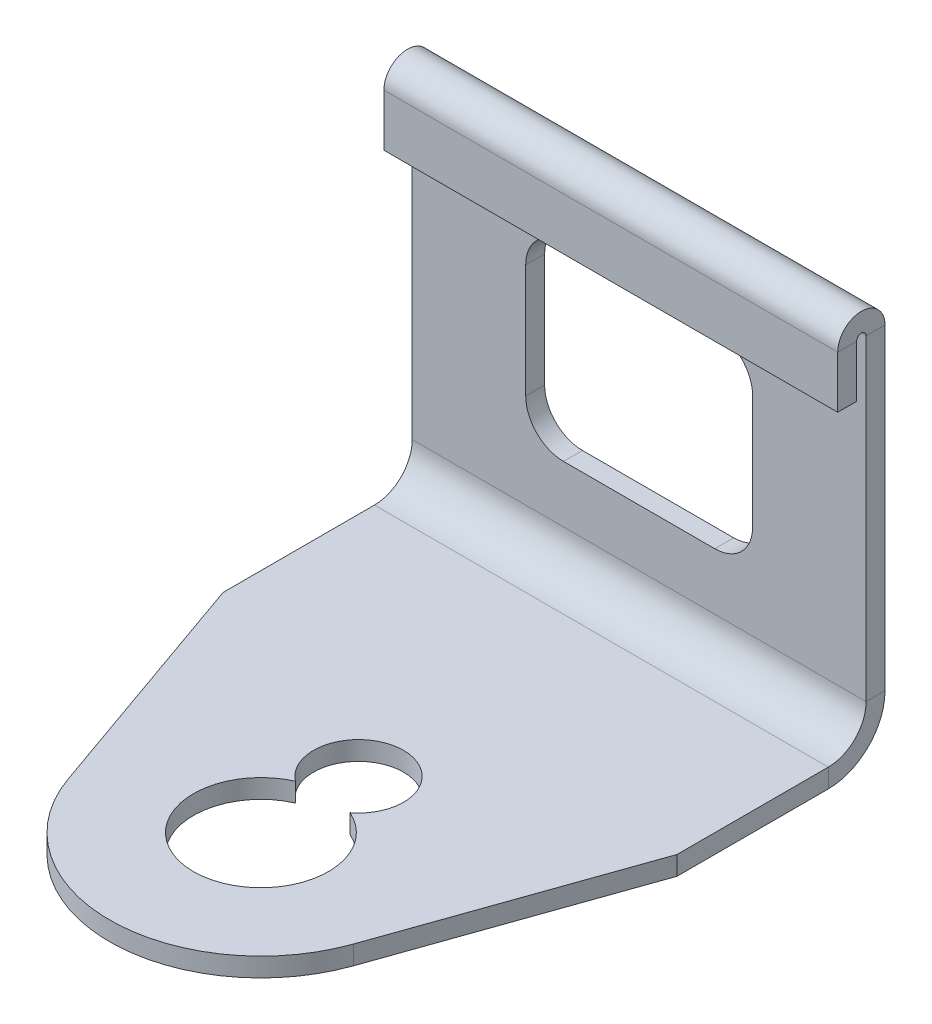
ISO-10303-21;
HEADER;
FILE_DESCRIPTION(('STEP AP214'),'2;1');
FILE_NAME('part.step','',(''),(''),'','','');
FILE_SCHEMA(('AUTOMOTIVE_DESIGN { 1 0 10303 214 1 1 1 1 }'));
ENDSEC;
DATA;
#1=APPLICATION_CONTEXT('core data for automotive mechanical design processes');
#2=APPLICATION_PROTOCOL_DEFINITION('international standard','automotive_design',2000,#1);
#3=PRODUCT_CONTEXT('',#1,'mechanical');
#4=PRODUCT('Part','Part','',(#3));
#5=PRODUCT_RELATED_PRODUCT_CATEGORY('part','',(#4));
#6=PRODUCT_DEFINITION_FORMATION('','',#4);
#7=PRODUCT_DEFINITION_CONTEXT('part definition',#1,'design');
#8=PRODUCT_DEFINITION('design','',#6,#7);
#9=PRODUCT_DEFINITION_SHAPE('','',#8);
#10=(LENGTH_UNIT() NAMED_UNIT(*) SI_UNIT(.MILLI.,.METRE.));
#11=(NAMED_UNIT(*) PLANE_ANGLE_UNIT() SI_UNIT($,.RADIAN.));
#12=(NAMED_UNIT(*) SI_UNIT($,.STERADIAN.) SOLID_ANGLE_UNIT());
#13=UNCERTAINTY_MEASURE_WITH_UNIT(LENGTH_MEASURE(1.E-05),#10,'distance_accuracy_value','');
#14=(GEOMETRIC_REPRESENTATION_CONTEXT(3) GLOBAL_UNCERTAINTY_ASSIGNED_CONTEXT((#13)) GLOBAL_UNIT_ASSIGNED_CONTEXT((#10,
#11,#12)) REPRESENTATION_CONTEXT('',''));
#15=CARTESIAN_POINT('',(0.,0.,0.));
#16=DIRECTION('',(0.,0.,1.));
#17=DIRECTION('',(1.,0.,0.));
#18=AXIS2_PLACEMENT_3D('',#15,#16,#17);
#19=CARTESIAN_POINT('',(-12.,-1.,11.));
#20=DIRECTION('',(-1.,0.,0.));
#21=DIRECTION('',(0.,0.,1.));
#22=AXIS2_PLACEMENT_3D('',#19,#20,#21);
#23=PLANE('',#22);
#24=DIRECTION('',(0.,0.,1.));
#25=VECTOR('',#24,1.);
#26=CARTESIAN_POINT('',(-12.,0.,11.));
#27=LINE('',#26,#25);
#28=CARTESIAN_POINT('',(-12.,0.,2.99999999999999));
#29=VERTEX_POINT('',#28);
#30=CARTESIAN_POINT('',(-12.,0.,11.));
#31=VERTEX_POINT('',#30);
#32=EDGE_CURVE('E463',#29,#31,#27,.T.);
#33=ORIENTED_EDGE('',*,*,#32,.F.);
#34=DIRECTION('',(0.,-1.,0.));
#35=VECTOR('',#34,1.);
#36=CARTESIAN_POINT('',(-12.,0.,2.99999999999999));
#37=LINE('',#36,#35);
#38=CARTESIAN_POINT('',(-12.,-1.00000000000002,2.99999999999999));
#39=VERTEX_POINT('',#38);
#40=EDGE_CURVE('E412',#29,#39,#37,.T.);
#41=ORIENTED_EDGE('',*,*,#40,.T.);
#42=DIRECTION('',(0.,0.,1.));
#43=VECTOR('',#42,1.);
#44=CARTESIAN_POINT('',(-12.,-1.,11.));
#45=LINE('',#44,#43);
#46=CARTESIAN_POINT('',(-12.,-1.,11.));
#47=VERTEX_POINT('',#46);
#48=EDGE_CURVE('E446',#39,#47,#45,.T.);
#49=ORIENTED_EDGE('',*,*,#48,.T.);
#50=DIRECTION('',(0.,1.,0.));
#51=VECTOR('',#50,1.);
#52=CARTESIAN_POINT('',(-12.,-1.,11.));
#53=LINE('',#52,#51);
#54=EDGE_CURVE('E97',#47,#31,#53,.T.);
#55=ORIENTED_EDGE('',*,*,#54,.T.);
#56=EDGE_LOOP('',(#33,#41,#49,#55));
#57=FACE_BOUND('',#56,.T.);
#58=ADVANCED_FACE('F92',(#57),#23,.T.);
#59=CARTESIAN_POINT('',(0.,-1.,21.));
#60=DIRECTION('',(0.,1.,0.));
#61=DIRECTION('',(0.,0.,1.));
#62=AXIS2_PLACEMENT_3D('',#59,#60,#61);
#63=PLANE('',#62);
#64=CARTESIAN_POINT('',(0.,-1.,15.84));
#65=DIRECTION('',(0.,1.,0.));
#66=DIRECTION('',(0.,0.,1.));
#67=AXIS2_PLACEMENT_3D('',#64,#65,#66);
#68=CIRCLE('',#67,2.38);
#69=CARTESIAN_POINT('',(1.44136175339873,-1.,17.7339050387597));
#70=VERTEX_POINT('',#69);
#71=CARTESIAN_POINT('',(-1.44136175339873,-1.,17.7339050387597));
#72=VERTEX_POINT('',#71);
#73=EDGE_CURVE('E435',#70,#72,#68,.T.);
#74=ORIENTED_EDGE('',*,*,#73,.T.);
#75=CARTESIAN_POINT('',(0.,-1.,21.));
#76=DIRECTION('',(0.,1.,0.));
#77=DIRECTION('',(0.,0.,1.));
#78=AXIS2_PLACEMENT_3D('',#75,#76,#77);
#79=CIRCLE('',#78,3.57);
#80=EDGE_CURVE('E427',#72,#70,#79,.T.);
#81=ORIENTED_EDGE('',*,*,#80,.T.);
#82=EDGE_LOOP('',(#74,#81));
#83=FACE_BOUND('',#82,.T.);
#84=DIRECTION('',(-1.,0.,0.));
#85=VECTOR('',#84,1.);
#86=CARTESIAN_POINT('',(-12.,-1.00000000000002,2.99999999999999));
#87=LINE('',#86,#85);
#88=CARTESIAN_POINT('',(12.,-1.,2.99999999999999));
#89=VERTEX_POINT('',#88);
#90=EDGE_CURVE('E406',#39,#89,#87,.F.);
#91=ORIENTED_EDGE('',*,*,#90,.T.);
#92=DIRECTION('',(0.,0.,-1.));
#93=VECTOR('',#92,1.);
#94=CARTESIAN_POINT('',(12.,-1.,11.));
#95=LINE('',#94,#93);
#96=CARTESIAN_POINT('',(12.,-1.,11.));
#97=VERTEX_POINT('',#96);
#98=EDGE_CURVE('E443',#97,#89,#95,.T.);
#99=ORIENTED_EDGE('',*,*,#98,.F.);
#100=DIRECTION('',(0.331954485163873,0.,-0.943295404303227));
#101=VECTOR('',#100,1.);
#102=CARTESIAN_POINT('',(12.,-1.,11.));
#103=LINE('',#102,#101);
#104=CARTESIAN_POINT('',(7.54636323442581,-1.,23.655635881311));
#105=VERTEX_POINT('',#104);
#106=EDGE_CURVE('E460',#105,#97,#103,.T.);
#107=ORIENTED_EDGE('',*,*,#106,.F.);
#108=CARTESIAN_POINT('',(0.,-1.,21.));
#109=DIRECTION('',(0.,1.,0.));
#110=DIRECTION('',(0.,0.,1.));
#111=AXIS2_PLACEMENT_3D('',#108,#109,#110);
#112=CIRCLE('',#111,8.);
#113=CARTESIAN_POINT('',(-7.54636323442581,-1.,23.655635881311));
#114=VERTEX_POINT('',#113);
#115=EDGE_CURVE('E455',#114,#105,#112,.T.);
#116=ORIENTED_EDGE('',*,*,#115,.F.);
#117=DIRECTION('',(0.331954485163873,0.,0.943295404303227));
#118=VECTOR('',#117,1.);
#119=CARTESIAN_POINT('',(-12.,-1.,11.));
#120=LINE('',#119,#118);
#121=EDGE_CURVE('E453',#47,#114,#120,.T.);
#122=ORIENTED_EDGE('',*,*,#121,.F.);
#123=ORIENTED_EDGE('',*,*,#48,.F.);
#124=EDGE_LOOP('',(#91,#99,#107,#116,#122,#123));
#125=FACE_BOUND('',#124,.T.);
#126=ADVANCED_FACE('F523',(#83,#125),#63,.F.);
#127=CARTESIAN_POINT('',(0.,0.,21.));
#128=DIRECTION('',(0.,1.,0.));
#129=DIRECTION('',(0.,0.,1.));
#130=AXIS2_PLACEMENT_3D('',#127,#128,#129);
#131=PLANE('',#130);
#132=CARTESIAN_POINT('',(0.,0.,21.));
#133=DIRECTION('',(0.,1.,0.));
#134=DIRECTION('',(0.,0.,1.));
#135=AXIS2_PLACEMENT_3D('',#132,#133,#134);
#136=CIRCLE('',#135,3.57);
#137=CARTESIAN_POINT('',(-1.44136175339873,0.,17.7339050387597));
#138=VERTEX_POINT('',#137);
#139=CARTESIAN_POINT('',(1.44136175339873,0.,17.7339050387597));
#140=VERTEX_POINT('',#139);
#141=EDGE_CURVE('E426',#138,#140,#136,.T.);
#142=ORIENTED_EDGE('',*,*,#141,.F.);
#143=CARTESIAN_POINT('',(0.,0.,15.84));
#144=DIRECTION('',(0.,1.,0.));
#145=DIRECTION('',(0.,0.,1.));
#146=AXIS2_PLACEMENT_3D('',#143,#144,#145);
#147=CIRCLE('',#146,2.38);
#148=EDGE_CURVE('E433',#140,#138,#147,.T.);
#149=ORIENTED_EDGE('',*,*,#148,.F.);
#150=EDGE_LOOP('',(#142,#149));
#151=FACE_BOUND('',#150,.T.);
#152=DIRECTION('',(0.,0.,-1.));
#153=VECTOR('',#152,1.);
#154=CARTESIAN_POINT('',(12.,0.,11.));
#155=LINE('',#154,#153);
#156=CARTESIAN_POINT('',(12.,0.,11.));
#157=VERTEX_POINT('',#156);
#158=CARTESIAN_POINT('',(12.,0.,2.99999999999999));
#159=VERTEX_POINT('',#158);
#160=EDGE_CURVE('E445',#157,#159,#155,.T.);
#161=ORIENTED_EDGE('',*,*,#160,.T.);
#162=DIRECTION('',(-1.,0.,0.));
#163=VECTOR('',#162,1.);
#164=CARTESIAN_POINT('',(-12.,0.,2.99999999999999));
#165=LINE('',#164,#163);
#166=EDGE_CURVE('E119',#29,#159,#165,.F.);
#167=ORIENTED_EDGE('',*,*,#166,.F.);
#168=ORIENTED_EDGE('',*,*,#32,.T.);
#169=DIRECTION('',(0.331954485163873,0.,0.943295404303227));
#170=VECTOR('',#169,1.);
#171=CARTESIAN_POINT('',(-12.,0.,11.));
#172=LINE('',#171,#170);
#173=CARTESIAN_POINT('',(-7.54636323442581,0.,23.655635881311));
#174=VERTEX_POINT('',#173);
#175=EDGE_CURVE('E461',#31,#174,#172,.T.);
#176=ORIENTED_EDGE('',*,*,#175,.T.);
#177=CARTESIAN_POINT('',(0.,0.,21.));
#178=DIRECTION('',(0.,1.,0.));
#179=DIRECTION('',(0.,0.,1.));
#180=AXIS2_PLACEMENT_3D('',#177,#178,#179);
#181=CIRCLE('',#180,8.);
#182=CARTESIAN_POINT('',(7.54636323442581,0.,23.655635881311));
#183=VERTEX_POINT('',#182);
#184=EDGE_CURVE('E468',#174,#183,#181,.T.);
#185=ORIENTED_EDGE('',*,*,#184,.T.);
#186=DIRECTION('',(0.331954485163873,0.,-0.943295404303227));
#187=VECTOR('',#186,1.);
#188=CARTESIAN_POINT('',(12.,0.,11.));
#189=LINE('',#188,#187);
#190=EDGE_CURVE('E447',#183,#157,#189,.T.);
#191=ORIENTED_EDGE('',*,*,#190,.T.);
#192=EDGE_LOOP('',(#161,#167,#168,#176,#185,#191));
#193=FACE_BOUND('',#192,.T.);
#194=ADVANCED_FACE('F481',(#151,#193),#131,.T.);
#195=CARTESIAN_POINT('',(12.,-1.,11.));
#196=DIRECTION('',(1.,0.,0.));
#197=DIRECTION('',(0.,0.,-1.));
#198=AXIS2_PLACEMENT_3D('',#195,#196,#197);
#199=PLANE('',#198);
#200=DIRECTION('',(0.,-1.,0.));
#201=VECTOR('',#200,1.);
#202=CARTESIAN_POINT('',(12.,0.,2.99999999999999));
#203=LINE('',#202,#201);
#204=EDGE_CURVE('E421',#159,#89,#203,.T.);
#205=ORIENTED_EDGE('',*,*,#204,.F.);
#206=ORIENTED_EDGE('',*,*,#160,.F.);
#207=DIRECTION('',(0.,1.,0.));
#208=VECTOR('',#207,1.);
#209=CARTESIAN_POINT('',(12.,-1.,11.));
#210=LINE('',#209,#208);
#211=EDGE_CURVE('E13',#97,#157,#210,.T.);
#212=ORIENTED_EDGE('',*,*,#211,.F.);
#213=ORIENTED_EDGE('',*,*,#98,.T.);
#214=EDGE_LOOP('',(#205,#206,#212,#213));
#215=FACE_BOUND('',#214,.T.);
#216=ADVANCED_FACE('F100',(#215),#199,.T.);
#217=CARTESIAN_POINT('',(12.,-1.,11.));
#218=DIRECTION('',(0.943295404303227,0.,0.331954485163873));
#219=DIRECTION('',(0.331954485163873,0.,-0.943295404303227));
#220=AXIS2_PLACEMENT_3D('',#217,#218,#219);
#221=PLANE('',#220);
#222=ORIENTED_EDGE('',*,*,#190,.F.);
#223=DIRECTION('',(0.,1.,0.));
#224=VECTOR('',#223,1.);
#225=CARTESIAN_POINT('',(7.54636323442581,-1.,23.655635881311));
#226=LINE('',#225,#224);
#227=EDGE_CURVE('E102',#105,#183,#226,.T.);
#228=ORIENTED_EDGE('',*,*,#227,.F.);
#229=ORIENTED_EDGE('',*,*,#106,.T.);
#230=ORIENTED_EDGE('',*,*,#211,.T.);
#231=EDGE_LOOP('',(#222,#228,#229,#230));
#232=FACE_BOUND('',#231,.T.);
#233=ADVANCED_FACE('F484',(#232),#221,.T.);
#234=CARTESIAN_POINT('',(0.,-1.,21.));
#235=DIRECTION('',(0.,1.,0.));
#236=DIRECTION('',(0.,0.,1.));
#237=AXIS2_PLACEMENT_3D('',#234,#235,#236);
#238=CYLINDRICAL_SURFACE('',#237,8.);
#239=ORIENTED_EDGE('',*,*,#184,.F.);
#240=DIRECTION('',(0.,1.,0.));
#241=VECTOR('',#240,1.);
#242=CARTESIAN_POINT('',(-7.54636323442581,-1.,23.655635881311));
#243=LINE('',#242,#241);
#244=EDGE_CURVE('E473',#114,#174,#243,.T.);
#245=ORIENTED_EDGE('',*,*,#244,.F.);
#246=ORIENTED_EDGE('',*,*,#115,.T.);
#247=ORIENTED_EDGE('',*,*,#227,.T.);
#248=EDGE_LOOP('',(#239,#245,#246,#247));
#249=FACE_BOUND('',#248,.T.);
#250=ADVANCED_FACE('F535',(#249),#238,.T.);
#251=CARTESIAN_POINT('',(-12.,-1.,11.));
#252=DIRECTION('',(-0.943295404303227,0.,0.331954485163873));
#253=DIRECTION('',(0.331954485163873,0.,0.943295404303227));
#254=AXIS2_PLACEMENT_3D('',#251,#252,#253);
#255=PLANE('',#254);
#256=ORIENTED_EDGE('',*,*,#175,.F.);
#257=ORIENTED_EDGE('',*,*,#54,.F.);
#258=ORIENTED_EDGE('',*,*,#121,.T.);
#259=ORIENTED_EDGE('',*,*,#244,.T.);
#260=EDGE_LOOP('',(#256,#257,#258,#259));
#261=FACE_BOUND('',#260,.T.);
#262=ADVANCED_FACE('F477',(#261),#255,.T.);
#263=CARTESIAN_POINT('',(0.,-1.,21.));
#264=DIRECTION('',(0.,1.,0.));
#265=DIRECTION('',(0.,0.,1.));
#266=AXIS2_PLACEMENT_3D('',#263,#264,#265);
#267=CYLINDRICAL_SURFACE('',#266,3.57);
#268=ORIENTED_EDGE('',*,*,#141,.T.);
#269=DIRECTION('',(0.,1.,0.));
#270=VECTOR('',#269,1.);
#271=CARTESIAN_POINT('',(1.44136175339873,-1.,17.7339050387597));
#272=LINE('',#271,#270);
#273=EDGE_CURVE('E436',#70,#140,#272,.T.);
#274=ORIENTED_EDGE('',*,*,#273,.F.);
#275=ORIENTED_EDGE('',*,*,#80,.F.);
#276=DIRECTION('',(0.,1.,0.));
#277=VECTOR('',#276,1.);
#278=CARTESIAN_POINT('',(-1.44136175339873,-1.,17.7339050387597));
#279=LINE('',#278,#277);
#280=EDGE_CURVE('E439',#72,#138,#279,.T.);
#281=ORIENTED_EDGE('',*,*,#280,.T.);
#282=EDGE_LOOP('',(#268,#274,#275,#281));
#283=FACE_BOUND('',#282,.T.);
#284=ADVANCED_FACE('F533',(#283),#267,.F.);
#285=CARTESIAN_POINT('',(0.,-1.,15.84));
#286=DIRECTION('',(0.,1.,0.));
#287=DIRECTION('',(0.,0.,1.));
#288=AXIS2_PLACEMENT_3D('',#285,#286,#287);
#289=CYLINDRICAL_SURFACE('',#288,2.38);
#290=ORIENTED_EDGE('',*,*,#148,.T.);
#291=ORIENTED_EDGE('',*,*,#280,.F.);
#292=ORIENTED_EDGE('',*,*,#73,.F.);
#293=ORIENTED_EDGE('',*,*,#273,.T.);
#294=EDGE_LOOP('',(#290,#291,#292,#293));
#295=FACE_BOUND('',#294,.T.);
#296=ADVANCED_FACE('F545',(#295),#289,.F.);
#297=CARTESIAN_POINT('',(12.,1.99999999999998,2.99999999999999));
#298=DIRECTION('',(1.,0.,0.));
#299=DIRECTION('',(0.,0.,-1.));
#300=AXIS2_PLACEMENT_3D('',#297,#298,#299);
#301=PLANE('',#300);
#302=DIRECTION('',(0.,0.,1.));
#303=VECTOR('',#302,1.);
#304=CARTESIAN_POINT('',(12.,2.,0.));
#305=LINE('',#304,#303);
#306=CARTESIAN_POINT('',(12.,1.99999999999997,0.999999999999993));
#307=VERTEX_POINT('',#306);
#308=CARTESIAN_POINT('',(12.,1.99999999999997,0.));
#309=VERTEX_POINT('',#308);
#310=EDGE_CURVE('E266',#307,#309,#305,.F.);
#311=ORIENTED_EDGE('',*,*,#310,.F.);
#312=CARTESIAN_POINT('',(12.,1.99999999999998,2.99999999999999));
#313=DIRECTION('',(-1.,0.,0.));
#314=DIRECTION('',(0.,0.,1.));
#315=AXIS2_PLACEMENT_3D('',#312,#313,#314);
#316=CIRCLE('',#315,2.);
#317=EDGE_CURVE('E417',#159,#307,#316,.F.);
#318=ORIENTED_EDGE('',*,*,#317,.F.);
#319=ORIENTED_EDGE('',*,*,#204,.T.);
#320=CARTESIAN_POINT('',(12.,1.99999999999998,2.99999999999999));
#321=DIRECTION('',(-1.,0.,0.));
#322=DIRECTION('',(0.,0.,1.));
#323=AXIS2_PLACEMENT_3D('',#320,#321,#322);
#324=CIRCLE('',#323,3.);
#325=EDGE_CURVE('E407',#89,#309,#324,.F.);
#326=ORIENTED_EDGE('',*,*,#325,.T.);
#327=EDGE_LOOP('',(#311,#318,#319,#326));
#328=FACE_BOUND('',#327,.T.);
#329=ADVANCED_FACE('F497',(#328),#301,.T.);
#330=CARTESIAN_POINT('',(-12.,1.99999999999998,2.99999999999999));
#331=DIRECTION('',(1.,0.,0.));
#332=DIRECTION('',(0.,0.,-1.));
#333=AXIS2_PLACEMENT_3D('',#330,#331,#332);
#334=PLANE('',#333);
#335=CARTESIAN_POINT('',(-12.,1.99999999999998,2.99999999999999));
#336=DIRECTION('',(-1.,0.,0.));
#337=DIRECTION('',(0.,0.,1.));
#338=AXIS2_PLACEMENT_3D('',#335,#336,#337);
#339=CIRCLE('',#338,2.);
#340=CARTESIAN_POINT('',(-12.,1.99999999999997,0.999999999999993));
#341=VERTEX_POINT('',#340);
#342=EDGE_CURVE('E358',#341,#29,#339,.T.);
#343=ORIENTED_EDGE('',*,*,#342,.F.);
#344=DIRECTION('',(0.,0.,1.));
#345=VECTOR('',#344,1.);
#346=CARTESIAN_POINT('',(-12.,1.99999999999999,0.999999999999993));
#347=LINE('',#346,#345);
#348=CARTESIAN_POINT('',(-12.,2.,0.));
#349=VERTEX_POINT('',#348);
#350=EDGE_CURVE('E405',#341,#349,#347,.F.);
#351=ORIENTED_EDGE('',*,*,#350,.T.);
#352=CARTESIAN_POINT('',(-12.,1.99999999999998,2.99999999999999));
#353=DIRECTION('',(-1.,0.,0.));
#354=DIRECTION('',(0.,0.,1.));
#355=AXIS2_PLACEMENT_3D('',#352,#353,#354);
#356=CIRCLE('',#355,3.);
#357=EDGE_CURVE('E413',#349,#39,#356,.T.);
#358=ORIENTED_EDGE('',*,*,#357,.T.);
#359=ORIENTED_EDGE('',*,*,#40,.F.);
#360=EDGE_LOOP('',(#343,#351,#358,#359));
#361=FACE_BOUND('',#360,.T.);
#362=ADVANCED_FACE('F501',(#361),#334,.F.);
#363=CARTESIAN_POINT('',(-12.,1.99999999999998,2.99999999999999));
#364=DIRECTION('',(-1.,0.,0.));
#365=DIRECTION('',(0.,0.,-1.));
#366=AXIS2_PLACEMENT_3D('',#363,#364,#365);
#367=CYLINDRICAL_SURFACE('',#366,3.);
#368=ORIENTED_EDGE('',*,*,#90,.F.);
#369=ORIENTED_EDGE('',*,*,#357,.F.);
#370=DIRECTION('',(-1.,0.,0.));
#371=VECTOR('',#370,1.);
#372=CARTESIAN_POINT('',(12.,2.,0.));
#373=LINE('',#372,#371);
#374=EDGE_CURVE('E396',#349,#309,#373,.F.);
#375=ORIENTED_EDGE('',*,*,#374,.T.);
#376=ORIENTED_EDGE('',*,*,#325,.F.);
#377=EDGE_LOOP('',(#368,#369,#375,#376));
#378=FACE_BOUND('',#377,.T.);
#379=ADVANCED_FACE('F498',(#378),#367,.T.);
#380=CARTESIAN_POINT('',(-12.,1.99999999999998,2.99999999999999));
#381=DIRECTION('',(-1.,0.,0.));
#382=DIRECTION('',(0.,0.,-1.));
#383=AXIS2_PLACEMENT_3D('',#380,#381,#382);
#384=CYLINDRICAL_SURFACE('',#383,2.);
#385=ORIENTED_EDGE('',*,*,#166,.T.);
#386=ORIENTED_EDGE('',*,*,#317,.T.);
#387=DIRECTION('',(-1.,0.,0.));
#388=VECTOR('',#387,1.);
#389=CARTESIAN_POINT('',(12.,1.99999999999999,0.999999999999993));
#390=LINE('',#389,#388);
#391=EDGE_CURVE('E403',#307,#341,#390,.T.);
#392=ORIENTED_EDGE('',*,*,#391,.T.);
#393=ORIENTED_EDGE('',*,*,#342,.T.);
#394=EDGE_LOOP('',(#385,#386,#392,#393));
#395=FACE_BOUND('',#394,.T.);
#396=ADVANCED_FACE('F495',(#395),#384,.F.);
#397=CARTESIAN_POINT('',(0.,0.,0.));
#398=DIRECTION('',(0.,0.,1.));
#399=DIRECTION('',(0.,-1.,0.));
#400=AXIS2_PLACEMENT_3D('',#397,#398,#399);
#401=PLANE('',#400);
#402=CARTESIAN_POINT('',(4.,7.,0.));
#403=DIRECTION('',(0.,0.,1.));
#404=DIRECTION('',(0.,-1.,0.));
#405=AXIS2_PLACEMENT_3D('',#402,#403,#404);
#406=CIRCLE('',#405,2.);
#407=CARTESIAN_POINT('',(6.,7.,0.));
#408=VERTEX_POINT('',#407);
#409=CARTESIAN_POINT('',(3.99999999999999,5.,0.));
#410=VERTEX_POINT('',#409);
#411=EDGE_CURVE('E372',#408,#410,#406,.F.);
#412=ORIENTED_EDGE('',*,*,#411,.F.);
#413=DIRECTION('',(0.,1.,0.));
#414=VECTOR('',#413,1.);
#415=CARTESIAN_POINT('',(6.,7.00000000000001,0.));
#416=LINE('',#415,#414);
#417=CARTESIAN_POINT('',(6.,13.,0.));
#418=VERTEX_POINT('',#417);
#419=EDGE_CURVE('E339',#418,#408,#416,.F.);
#420=ORIENTED_EDGE('',*,*,#419,.F.);
#421=CARTESIAN_POINT('',(4.,13.,0.));
#422=DIRECTION('',(0.,0.,1.));
#423=DIRECTION('',(0.,-1.,0.));
#424=AXIS2_PLACEMENT_3D('',#421,#422,#423);
#425=CIRCLE('',#424,2.);
#426=CARTESIAN_POINT('',(3.99999999999999,15.,0.));
#427=VERTEX_POINT('',#426);
#428=EDGE_CURVE('E363',#427,#418,#425,.F.);
#429=ORIENTED_EDGE('',*,*,#428,.F.);
#430=DIRECTION('',(-1.,0.,0.));
#431=VECTOR('',#430,1.);
#432=CARTESIAN_POINT('',(3.99999999999998,15.,0.));
#433=LINE('',#432,#431);
#434=CARTESIAN_POINT('',(-3.99999999999999,15.,0.));
#435=VERTEX_POINT('',#434);
#436=EDGE_CURVE('E365',#435,#427,#433,.F.);
#437=ORIENTED_EDGE('',*,*,#436,.F.);
#438=CARTESIAN_POINT('',(-4.,13.,0.));
#439=DIRECTION('',(0.,0.,1.));
#440=DIRECTION('',(0.,-1.,0.));
#441=AXIS2_PLACEMENT_3D('',#438,#439,#440);
#442=CIRCLE('',#441,2.);
#443=CARTESIAN_POINT('',(-6.,13.,0.));
#444=VERTEX_POINT('',#443);
#445=EDGE_CURVE('E368',#444,#435,#442,.F.);
#446=ORIENTED_EDGE('',*,*,#445,.F.);
#447=DIRECTION('',(0.,-1.,0.));
#448=VECTOR('',#447,1.);
#449=CARTESIAN_POINT('',(-6.,7.00000000000001,0.));
#450=LINE('',#449,#448);
#451=CARTESIAN_POINT('',(-6.,7.,0.));
#452=VERTEX_POINT('',#451);
#453=EDGE_CURVE('E366',#452,#444,#450,.F.);
#454=ORIENTED_EDGE('',*,*,#453,.F.);
#455=CARTESIAN_POINT('',(-4.,7.,0.));
#456=DIRECTION('',(0.,0.,1.));
#457=DIRECTION('',(0.,-1.,0.));
#458=AXIS2_PLACEMENT_3D('',#455,#456,#457);
#459=CIRCLE('',#458,2.);
#460=CARTESIAN_POINT('',(-3.99999999999999,5.,0.));
#461=VERTEX_POINT('',#460);
#462=EDGE_CURVE('E367',#461,#452,#459,.F.);
#463=ORIENTED_EDGE('',*,*,#462,.F.);
#464=DIRECTION('',(1.,0.,0.));
#465=VECTOR('',#464,1.);
#466=CARTESIAN_POINT('',(3.99999999999998,5.,0.));
#467=LINE('',#466,#465);
#468=EDGE_CURVE('E375',#410,#461,#467,.F.);
#469=ORIENTED_EDGE('',*,*,#468,.F.);
#470=EDGE_LOOP('',(#412,#420,#429,#437,#446,#454,#463,#469));
#471=FACE_BOUND('',#470,.T.);
#472=DIRECTION('',(0.,1.,0.));
#473=VECTOR('',#472,1.);
#474=CARTESIAN_POINT('',(-12.,0.,0.));
#475=LINE('',#474,#473);
#476=CARTESIAN_POINT('',(-12.,18.75,0.));
#477=VERTEX_POINT('',#476);
#478=EDGE_CURVE('E269',#349,#477,#475,.T.);
#479=ORIENTED_EDGE('',*,*,#478,.T.);
#480=DIRECTION('',(-1.,0.,0.));
#481=VECTOR('',#480,1.);
#482=CARTESIAN_POINT('',(-12.,18.75,0.));
#483=LINE('',#482,#481);
#484=CARTESIAN_POINT('',(12.,18.75,0.));
#485=VERTEX_POINT('',#484);
#486=EDGE_CURVE('E273',#477,#485,#483,.F.);
#487=ORIENTED_EDGE('',*,*,#486,.T.);
#488=DIRECTION('',(0.,-1.,0.));
#489=VECTOR('',#488,1.);
#490=CARTESIAN_POINT('',(12.,0.,0.));
#491=LINE('',#490,#489);
#492=EDGE_CURVE('E259',#485,#309,#491,.T.);
#493=ORIENTED_EDGE('',*,*,#492,.T.);
#494=ORIENTED_EDGE('',*,*,#374,.F.);
#495=EDGE_LOOP('',(#479,#487,#493,#494));
#496=FACE_BOUND('',#495,.T.);
#497=ADVANCED_FACE('F274',(#471,#496),#401,.F.);
#498=CARTESIAN_POINT('',(0.,0.,1.));
#499=DIRECTION('',(0.,0.,1.));
#500=DIRECTION('',(0.,-1.,0.));
#501=AXIS2_PLACEMENT_3D('',#498,#499,#500);
#502=PLANE('',#501);
#503=DIRECTION('',(-1.,0.,0.));
#504=VECTOR('',#503,1.);
#505=CARTESIAN_POINT('',(-12.,18.75,0.999999999999934));
#506=LINE('',#505,#504);
#507=CARTESIAN_POINT('',(-12.,18.75,0.999999999999934));
#508=VERTEX_POINT('',#507);
#509=CARTESIAN_POINT('',(12.,18.75,0.999999999999934));
#510=VERTEX_POINT('',#509);
#511=EDGE_CURVE('E297',#508,#510,#506,.F.);
#512=ORIENTED_EDGE('',*,*,#511,.F.);
#513=DIRECTION('',(0.,-1.,0.));
#514=VECTOR('',#513,1.);
#515=CARTESIAN_POINT('',(-12.,20.,0.99999999999993));
#516=LINE('',#515,#514);
#517=EDGE_CURVE('E271',#341,#508,#516,.F.);
#518=ORIENTED_EDGE('',*,*,#517,.F.);
#519=ORIENTED_EDGE('',*,*,#391,.F.);
#520=DIRECTION('',(0.,1.,0.));
#521=VECTOR('',#520,1.);
#522=CARTESIAN_POINT('',(12.,0.,1.));
#523=LINE('',#522,#521);
#524=EDGE_CURVE('E352',#510,#307,#523,.F.);
#525=ORIENTED_EDGE('',*,*,#524,.F.);
#526=EDGE_LOOP('',(#512,#518,#519,#525));
#527=FACE_BOUND('',#526,.T.);
#528=DIRECTION('',(0.,-1.,0.));
#529=VECTOR('',#528,1.);
#530=CARTESIAN_POINT('',(6.,0.,1.));
#531=LINE('',#530,#529);
#532=CARTESIAN_POINT('',(6.,13.,0.999999999999955));
#533=VERTEX_POINT('',#532);
#534=CARTESIAN_POINT('',(6.,7.00000000000001,0.999999999999975));
#535=VERTEX_POINT('',#534);
#536=EDGE_CURVE('E376',#533,#535,#531,.T.);
#537=ORIENTED_EDGE('',*,*,#536,.T.);
#538=CARTESIAN_POINT('',(4.,7.,0.999999999999975));
#539=DIRECTION('',(0.,0.,1.));
#540=DIRECTION('',(0.,-1.,0.));
#541=AXIS2_PLACEMENT_3D('',#538,#539,#540);
#542=CIRCLE('',#541,2.);
#543=CARTESIAN_POINT('',(3.99999999999999,5.,0.999999999999982));
#544=VERTEX_POINT('',#543);
#545=EDGE_CURVE('E399',#535,#544,#542,.F.);
#546=ORIENTED_EDGE('',*,*,#545,.T.);
#547=DIRECTION('',(-1.,0.,0.));
#548=VECTOR('',#547,1.);
#549=CARTESIAN_POINT('',(0.,5.,0.999999999999982));
#550=LINE('',#549,#548);
#551=CARTESIAN_POINT('',(-3.99999999999999,5.,0.999999999999982));
#552=VERTEX_POINT('',#551);
#553=EDGE_CURVE('E392',#544,#552,#550,.T.);
#554=ORIENTED_EDGE('',*,*,#553,.T.);
#555=CARTESIAN_POINT('',(-4.,7.,0.999999999999975));
#556=DIRECTION('',(0.,0.,1.));
#557=DIRECTION('',(0.,-1.,0.));
#558=AXIS2_PLACEMENT_3D('',#555,#556,#557);
#559=CIRCLE('',#558,2.);
#560=CARTESIAN_POINT('',(-6.,7.00000000000001,0.999999999999975));
#561=VERTEX_POINT('',#560);
#562=EDGE_CURVE('E393',#552,#561,#559,.F.);
#563=ORIENTED_EDGE('',*,*,#562,.T.);
#564=DIRECTION('',(0.,1.,0.));
#565=VECTOR('',#564,1.);
#566=CARTESIAN_POINT('',(-6.,0.,1.));
#567=LINE('',#566,#565);
#568=CARTESIAN_POINT('',(-6.,13.,0.999999999999955));
#569=VERTEX_POINT('',#568);
#570=EDGE_CURVE('E389',#561,#569,#567,.T.);
#571=ORIENTED_EDGE('',*,*,#570,.T.);
#572=CARTESIAN_POINT('',(-4.,13.,0.999999999999955));
#573=DIRECTION('',(0.,0.,1.));
#574=DIRECTION('',(0.,-1.,0.));
#575=AXIS2_PLACEMENT_3D('',#572,#573,#574);
#576=CIRCLE('',#575,2.);
#577=CARTESIAN_POINT('',(-3.99999999999999,15.,0.999999999999948));
#578=VERTEX_POINT('',#577);
#579=EDGE_CURVE('E384',#569,#578,#576,.F.);
#580=ORIENTED_EDGE('',*,*,#579,.T.);
#581=DIRECTION('',(1.,0.,0.));
#582=VECTOR('',#581,1.);
#583=CARTESIAN_POINT('',(0.,15.,0.999999999999948));
#584=LINE('',#583,#582);
#585=CARTESIAN_POINT('',(3.99999999999999,15.,0.999999999999948));
#586=VERTEX_POINT('',#585);
#587=EDGE_CURVE('E385',#578,#586,#584,.T.);
#588=ORIENTED_EDGE('',*,*,#587,.T.);
#589=CARTESIAN_POINT('',(4.,13.,0.999999999999955));
#590=DIRECTION('',(0.,0.,1.));
#591=DIRECTION('',(0.,-1.,0.));
#592=AXIS2_PLACEMENT_3D('',#589,#590,#591);
#593=CIRCLE('',#592,2.);
#594=EDGE_CURVE('E377',#586,#533,#593,.F.);
#595=ORIENTED_EDGE('',*,*,#594,.T.);
#596=EDGE_LOOP('',(#537,#546,#554,#563,#571,#580,#588,#595));
#597=FACE_BOUND('',#596,.T.);
#598=ADVANCED_FACE('F520',(#527,#597),#502,.T.);
#599=CARTESIAN_POINT('',(12.,0.,0.));
#600=DIRECTION('',(-1.,0.,0.));
#601=DIRECTION('',(0.,0.,1.));
#602=AXIS2_PLACEMENT_3D('',#599,#600,#601);
#603=PLANE('',#602);
#604=ORIENTED_EDGE('',*,*,#492,.F.);
#605=DIRECTION('',(0.,0.,-1.));
#606=VECTOR('',#605,1.);
#607=CARTESIAN_POINT('',(12.,18.75,0.999999999999934));
#608=LINE('',#607,#606);
#609=EDGE_CURVE('E263',#510,#485,#608,.T.);
#610=ORIENTED_EDGE('',*,*,#609,.F.);
#611=ORIENTED_EDGE('',*,*,#524,.T.);
#612=ORIENTED_EDGE('',*,*,#310,.T.);
#613=EDGE_LOOP('',(#604,#610,#611,#612));
#614=FACE_BOUND('',#613,.T.);
#615=ADVANCED_FACE('F261',(#614),#603,.F.);
#616=CARTESIAN_POINT('',(-12.,20.,0.));
#617=DIRECTION('',(1.,0.,0.));
#618=DIRECTION('',(0.,0.,-1.));
#619=AXIS2_PLACEMENT_3D('',#616,#617,#618);
#620=PLANE('',#619);
#621=ORIENTED_EDGE('',*,*,#517,.T.);
#622=DIRECTION('',(0.,0.,-1.));
#623=VECTOR('',#622,1.);
#624=CARTESIAN_POINT('',(-12.,18.75,0.999999999999934));
#625=LINE('',#624,#623);
#626=EDGE_CURVE('E115',#508,#477,#625,.T.);
#627=ORIENTED_EDGE('',*,*,#626,.T.);
#628=ORIENTED_EDGE('',*,*,#478,.F.);
#629=ORIENTED_EDGE('',*,*,#350,.F.);
#630=EDGE_LOOP('',(#621,#627,#628,#629));
#631=FACE_BOUND('',#630,.T.);
#632=ADVANCED_FACE('F504',(#631),#620,.F.);
#633=CARTESIAN_POINT('',(4.,7.,0.));
#634=DIRECTION('',(0.,0.,1.));
#635=DIRECTION('',(0.,-1.,0.));
#636=AXIS2_PLACEMENT_3D('',#633,#634,#635);
#637=CYLINDRICAL_SURFACE('',#636,2.);
#638=ORIENTED_EDGE('',*,*,#545,.F.);
#639=DIRECTION('',(0.,0.,1.));
#640=VECTOR('',#639,1.);
#641=CARTESIAN_POINT('',(6.,7.00000000000001,0.));
#642=LINE('',#641,#640);
#643=EDGE_CURVE('E338',#408,#535,#642,.T.);
#644=ORIENTED_EDGE('',*,*,#643,.F.);
#645=ORIENTED_EDGE('',*,*,#411,.T.);
#646=DIRECTION('',(0.,0.,1.));
#647=VECTOR('',#646,1.);
#648=CARTESIAN_POINT('',(3.99999999999998,5.,0.));
#649=LINE('',#648,#647);
#650=EDGE_CURVE('E355',#410,#544,#649,.T.);
#651=ORIENTED_EDGE('',*,*,#650,.T.);
#652=EDGE_LOOP('',(#638,#644,#645,#651));
#653=FACE_BOUND('',#652,.T.);
#654=ADVANCED_FACE('F509',(#653),#637,.F.);
#655=CARTESIAN_POINT('',(3.99999999999998,5.,0.));
#656=DIRECTION('',(0.,1.,0.));
#657=DIRECTION('',(0.,0.,1.));
#658=AXIS2_PLACEMENT_3D('',#655,#656,#657);
#659=PLANE('',#658);
#660=ORIENTED_EDGE('',*,*,#553,.F.);
#661=ORIENTED_EDGE('',*,*,#650,.F.);
#662=ORIENTED_EDGE('',*,*,#468,.T.);
#663=DIRECTION('',(0.,0.,1.));
#664=VECTOR('',#663,1.);
#665=CARTESIAN_POINT('',(-3.99999999999999,5.,0.));
#666=LINE('',#665,#664);
#667=EDGE_CURVE('E348',#461,#552,#666,.T.);
#668=ORIENTED_EDGE('',*,*,#667,.T.);
#669=EDGE_LOOP('',(#660,#661,#662,#668));
#670=FACE_BOUND('',#669,.T.);
#671=ADVANCED_FACE('F514',(#670),#659,.T.);
#672=CARTESIAN_POINT('',(-4.,7.,0.));
#673=DIRECTION('',(0.,0.,1.));
#674=DIRECTION('',(0.,-1.,0.));
#675=AXIS2_PLACEMENT_3D('',#672,#673,#674);
#676=CYLINDRICAL_SURFACE('',#675,2.);
#677=ORIENTED_EDGE('',*,*,#562,.F.);
#678=ORIENTED_EDGE('',*,*,#667,.F.);
#679=ORIENTED_EDGE('',*,*,#462,.T.);
#680=DIRECTION('',(0.,0.,1.));
#681=VECTOR('',#680,1.);
#682=CARTESIAN_POINT('',(-6.,7.00000000000001,0.));
#683=LINE('',#682,#681);
#684=EDGE_CURVE('E346',#452,#561,#683,.T.);
#685=ORIENTED_EDGE('',*,*,#684,.T.);
#686=EDGE_LOOP('',(#677,#678,#679,#685));
#687=FACE_BOUND('',#686,.T.);
#688=ADVANCED_FACE('F572',(#687),#676,.F.);
#689=CARTESIAN_POINT('',(-6.,7.00000000000001,0.));
#690=DIRECTION('',(1.,0.,0.));
#691=DIRECTION('',(0.,0.,-1.));
#692=AXIS2_PLACEMENT_3D('',#689,#690,#691);
#693=PLANE('',#692);
#694=ORIENTED_EDGE('',*,*,#570,.F.);
#695=ORIENTED_EDGE('',*,*,#684,.F.);
#696=ORIENTED_EDGE('',*,*,#453,.T.);
#697=DIRECTION('',(0.,0.,1.));
#698=VECTOR('',#697,1.);
#699=CARTESIAN_POINT('',(-6.,13.,0.));
#700=LINE('',#699,#698);
#701=EDGE_CURVE('E347',#444,#569,#700,.T.);
#702=ORIENTED_EDGE('',*,*,#701,.T.);
#703=EDGE_LOOP('',(#694,#695,#696,#702));
#704=FACE_BOUND('',#703,.T.);
#705=ADVANCED_FACE('F585',(#704),#693,.T.);
#706=CARTESIAN_POINT('',(-4.,13.,0.));
#707=DIRECTION('',(0.,0.,1.));
#708=DIRECTION('',(0.,-1.,0.));
#709=AXIS2_PLACEMENT_3D('',#706,#707,#708);
#710=CYLINDRICAL_SURFACE('',#709,2.);
#711=ORIENTED_EDGE('',*,*,#579,.F.);
#712=ORIENTED_EDGE('',*,*,#701,.F.);
#713=ORIENTED_EDGE('',*,*,#445,.T.);
#714=DIRECTION('',(0.,0.,1.));
#715=VECTOR('',#714,1.);
#716=CARTESIAN_POINT('',(-3.99999999999999,15.,0.));
#717=LINE('',#716,#715);
#718=EDGE_CURVE('E345',#435,#578,#717,.T.);
#719=ORIENTED_EDGE('',*,*,#718,.T.);
#720=EDGE_LOOP('',(#711,#712,#713,#719));
#721=FACE_BOUND('',#720,.T.);
#722=ADVANCED_FACE('F593',(#721),#710,.F.);
#723=CARTESIAN_POINT('',(3.99999999999998,15.,0.));
#724=DIRECTION('',(0.,-1.,0.));
#725=DIRECTION('',(0.,0.,-1.));
#726=AXIS2_PLACEMENT_3D('',#723,#724,#725);
#727=PLANE('',#726);
#728=ORIENTED_EDGE('',*,*,#587,.F.);
#729=ORIENTED_EDGE('',*,*,#718,.F.);
#730=ORIENTED_EDGE('',*,*,#436,.T.);
#731=DIRECTION('',(0.,0.,1.));
#732=VECTOR('',#731,1.);
#733=CARTESIAN_POINT('',(3.99999999999998,15.,0.));
#734=LINE('',#733,#732);
#735=EDGE_CURVE('E344',#427,#586,#734,.T.);
#736=ORIENTED_EDGE('',*,*,#735,.T.);
#737=EDGE_LOOP('',(#728,#729,#730,#736));
#738=FACE_BOUND('',#737,.T.);
#739=ADVANCED_FACE('F605',(#738),#727,.T.);
#740=CARTESIAN_POINT('',(4.,13.,0.));
#741=DIRECTION('',(0.,0.,1.));
#742=DIRECTION('',(0.,-1.,0.));
#743=AXIS2_PLACEMENT_3D('',#740,#741,#742);
#744=CYLINDRICAL_SURFACE('',#743,2.);
#745=ORIENTED_EDGE('',*,*,#594,.F.);
#746=ORIENTED_EDGE('',*,*,#735,.F.);
#747=ORIENTED_EDGE('',*,*,#428,.T.);
#748=DIRECTION('',(0.,0.,1.));
#749=VECTOR('',#748,1.);
#750=CARTESIAN_POINT('',(6.,13.,0.));
#751=LINE('',#750,#749);
#752=EDGE_CURVE('E337',#418,#533,#751,.T.);
#753=ORIENTED_EDGE('',*,*,#752,.T.);
#754=EDGE_LOOP('',(#745,#746,#747,#753));
#755=FACE_BOUND('',#754,.T.);
#756=ADVANCED_FACE('F613',(#755),#744,.F.);
#757=CARTESIAN_POINT('',(6.,7.00000000000001,0.));
#758=DIRECTION('',(-1.,0.,0.));
#759=DIRECTION('',(0.,0.,1.));
#760=AXIS2_PLACEMENT_3D('',#757,#758,#759);
#761=PLANE('',#760);
#762=ORIENTED_EDGE('',*,*,#536,.F.);
#763=ORIENTED_EDGE('',*,*,#752,.F.);
#764=ORIENTED_EDGE('',*,*,#419,.T.);
#765=ORIENTED_EDGE('',*,*,#643,.T.);
#766=EDGE_LOOP('',(#762,#763,#764,#765));
#767=FACE_BOUND('',#766,.T.);
#768=ADVANCED_FACE('F616',(#767),#761,.T.);
#769=CARTESIAN_POINT('',(-12.,17.375,2.49999999999994));
#770=DIRECTION('',(1.,0.,0.));
#771=DIRECTION('',(0.,1.,0.));
#772=AXIS2_PLACEMENT_3D('',#769,#770,#771);
#773=PLANE('',#772);
#774=DIRECTION('',(0.,0.,1.));
#775=VECTOR('',#774,1.);
#776=CARTESIAN_POINT('',(-12.,18.75,2.49999999999993));
#777=LINE('',#776,#775);
#778=CARTESIAN_POINT('',(-12.,18.75,1.49999999999993));
#779=VERTEX_POINT('',#778);
#780=CARTESIAN_POINT('',(-12.,18.75,2.49999999999993));
#781=VERTEX_POINT('',#780);
#782=EDGE_CURVE('E328',#779,#781,#777,.T.);
#783=ORIENTED_EDGE('',*,*,#782,.F.);
#784=DIRECTION('',(0.,-1.,0.));
#785=VECTOR('',#784,1.);
#786=CARTESIAN_POINT('',(-12.,17.375,1.49999999999994));
#787=LINE('',#786,#785);
#788=CARTESIAN_POINT('',(-12.,16.,1.49999999999994));
#789=VERTEX_POINT('',#788);
#790=EDGE_CURVE('E319',#789,#779,#787,.F.);
#791=ORIENTED_EDGE('',*,*,#790,.F.);
#792=DIRECTION('',(0.,0.,1.));
#793=VECTOR('',#792,1.);
#794=CARTESIAN_POINT('',(-12.,16.,2.49999999999994));
#795=LINE('',#794,#793);
#796=CARTESIAN_POINT('',(-12.,16.,2.49999999999994));
#797=VERTEX_POINT('',#796);
#798=EDGE_CURVE('E330',#789,#797,#795,.T.);
#799=ORIENTED_EDGE('',*,*,#798,.T.);
#800=DIRECTION('',(0.,1.,0.));
#801=VECTOR('',#800,1.);
#802=CARTESIAN_POINT('',(-12.,17.375,2.49999999999994));
#803=LINE('',#802,#801);
#804=EDGE_CURVE('E309',#797,#781,#803,.T.);
#805=ORIENTED_EDGE('',*,*,#804,.T.);
#806=EDGE_LOOP('',(#783,#791,#799,#805));
#807=FACE_BOUND('',#806,.T.);
#808=ADVANCED_FACE('F629',(#807),#773,.F.);
#809=CARTESIAN_POINT('',(0.,16.,2.49999999999994));
#810=DIRECTION('',(0.,1.,0.));
#811=DIRECTION('',(-1.,0.,0.));
#812=AXIS2_PLACEMENT_3D('',#809,#810,#811);
#813=PLANE('',#812);
#814=ORIENTED_EDGE('',*,*,#798,.F.);
#815=DIRECTION('',(1.,0.,0.));
#816=VECTOR('',#815,1.);
#817=CARTESIAN_POINT('',(0.,16.,1.49999999999994));
#818=LINE('',#817,#816);
#819=CARTESIAN_POINT('',(12.,16.,1.49999999999994));
#820=VERTEX_POINT('',#819);
#821=EDGE_CURVE('E320',#820,#789,#818,.F.);
#822=ORIENTED_EDGE('',*,*,#821,.F.);
#823=DIRECTION('',(0.,0.,1.));
#824=VECTOR('',#823,1.);
#825=CARTESIAN_POINT('',(12.,16.,2.49999999999994));
#826=LINE('',#825,#824);
#827=CARTESIAN_POINT('',(12.,16.,2.49999999999994));
#828=VERTEX_POINT('',#827);
#829=EDGE_CURVE('E310',#820,#828,#826,.T.);
#830=ORIENTED_EDGE('',*,*,#829,.T.);
#831=DIRECTION('',(-1.,0.,0.));
#832=VECTOR('',#831,1.);
#833=CARTESIAN_POINT('',(0.,16.,2.49999999999994));
#834=LINE('',#833,#832);
#835=EDGE_CURVE('E308',#828,#797,#834,.T.);
#836=ORIENTED_EDGE('',*,*,#835,.T.);
#837=EDGE_LOOP('',(#814,#822,#830,#836));
#838=FACE_BOUND('',#837,.T.);
#839=ADVANCED_FACE('F689',(#838),#813,.F.);
#840=CARTESIAN_POINT('',(12.,17.375,2.49999999999994));
#841=DIRECTION('',(-1.,0.,0.));
#842=DIRECTION('',(0.,-1.,0.));
#843=AXIS2_PLACEMENT_3D('',#840,#841,#842);
#844=PLANE('',#843);
#845=DIRECTION('',(0.,-1.,0.));
#846=VECTOR('',#845,1.);
#847=CARTESIAN_POINT('',(12.,17.375,1.49999999999994));
#848=LINE('',#847,#846);
#849=CARTESIAN_POINT('',(12.,18.75,1.49999999999993));
#850=VERTEX_POINT('',#849);
#851=EDGE_CURVE('E286',#850,#820,#848,.T.);
#852=ORIENTED_EDGE('',*,*,#851,.F.);
#853=DIRECTION('',(0.,0.,1.));
#854=VECTOR('',#853,1.);
#855=CARTESIAN_POINT('',(12.,18.75,2.49999999999993));
#856=LINE('',#855,#854);
#857=CARTESIAN_POINT('',(12.,18.75,2.49999999999993));
#858=VERTEX_POINT('',#857);
#859=EDGE_CURVE('E335',#850,#858,#856,.T.);
#860=ORIENTED_EDGE('',*,*,#859,.T.);
#861=DIRECTION('',(0.,-1.,0.));
#862=VECTOR('',#861,1.);
#863=CARTESIAN_POINT('',(12.,17.375,2.49999999999994));
#864=LINE('',#863,#862);
#865=EDGE_CURVE('E314',#858,#828,#864,.T.);
#866=ORIENTED_EDGE('',*,*,#865,.T.);
#867=ORIENTED_EDGE('',*,*,#829,.F.);
#868=EDGE_LOOP('',(#852,#860,#866,#867));
#869=FACE_BOUND('',#868,.T.);
#870=ADVANCED_FACE('F701',(#869),#844,.F.);
#871=CARTESIAN_POINT('',(0.,17.375,2.49999999999994));
#872=DIRECTION('',(0.,0.,1.));
#873=DIRECTION('',(0.,-1.,0.));
#874=AXIS2_PLACEMENT_3D('',#871,#872,#873);
#875=PLANE('',#874);
#876=ORIENTED_EDGE('',*,*,#835,.F.);
#877=ORIENTED_EDGE('',*,*,#865,.F.);
#878=DIRECTION('',(1.,0.,0.));
#879=VECTOR('',#878,1.);
#880=CARTESIAN_POINT('',(0.,18.75,2.49999999999993));
#881=LINE('',#880,#879);
#882=EDGE_CURVE('E294',#781,#858,#881,.T.);
#883=ORIENTED_EDGE('',*,*,#882,.F.);
#884=ORIENTED_EDGE('',*,*,#804,.F.);
#885=EDGE_LOOP('',(#876,#877,#883,#884));
#886=FACE_BOUND('',#885,.T.);
#887=ADVANCED_FACE('F715',(#886),#875,.T.);
#888=CARTESIAN_POINT('',(0.,17.375,1.49999999999994));
#889=DIRECTION('',(0.,0.,1.));
#890=DIRECTION('',(0.,-1.,0.));
#891=AXIS2_PLACEMENT_3D('',#888,#889,#890);
#892=PLANE('',#891);
#893=ORIENTED_EDGE('',*,*,#821,.T.);
#894=ORIENTED_EDGE('',*,*,#790,.T.);
#895=DIRECTION('',(1.,0.,0.));
#896=VECTOR('',#895,1.);
#897=CARTESIAN_POINT('',(0.,18.75,1.49999999999993));
#898=LINE('',#897,#896);
#899=EDGE_CURVE('E323',#779,#850,#898,.T.);
#900=ORIENTED_EDGE('',*,*,#899,.T.);
#901=ORIENTED_EDGE('',*,*,#851,.T.);
#902=EDGE_LOOP('',(#893,#894,#900,#901));
#903=FACE_BOUND('',#902,.T.);
#904=ADVANCED_FACE('F721',(#903),#892,.F.);
#905=CARTESIAN_POINT('',(12.,18.75,1.24999999999993));
#906=DIRECTION('',(1.,0.,0.));
#907=DIRECTION('',(0.,0.,-1.));
#908=AXIS2_PLACEMENT_3D('',#905,#906,#907);
#909=PLANE('',#908);
#910=ORIENTED_EDGE('',*,*,#859,.F.);
#911=CARTESIAN_POINT('',(12.,18.75,1.24999999999993));
#912=DIRECTION('',(-1.,0.,0.));
#913=DIRECTION('',(0.,0.,1.));
#914=AXIS2_PLACEMENT_3D('',#911,#912,#913);
#915=CIRCLE('',#914,0.25);
#916=EDGE_CURVE('E290',#510,#850,#915,.F.);
#917=ORIENTED_EDGE('',*,*,#916,.F.);
#918=ORIENTED_EDGE('',*,*,#609,.T.);
#919=CARTESIAN_POINT('',(12.,18.75,1.24999999999993));
#920=DIRECTION('',(-1.,0.,0.));
#921=DIRECTION('',(0.,0.,1.));
#922=AXIS2_PLACEMENT_3D('',#919,#920,#921);
#923=CIRCLE('',#922,1.25);
#924=EDGE_CURVE('E278',#485,#858,#923,.F.);
#925=ORIENTED_EDGE('',*,*,#924,.T.);
#926=EDGE_LOOP('',(#910,#917,#918,#925));
#927=FACE_BOUND('',#926,.T.);
#928=ADVANCED_FACE('F289',(#927),#909,.T.);
#929=CARTESIAN_POINT('',(-12.,18.75,1.24999999999993));
#930=DIRECTION('',(1.,0.,0.));
#931=DIRECTION('',(0.,0.,-1.));
#932=AXIS2_PLACEMENT_3D('',#929,#930,#931);
#933=PLANE('',#932);
#934=CARTESIAN_POINT('',(-12.,18.75,1.24999999999993));
#935=DIRECTION('',(-1.,0.,0.));
#936=DIRECTION('',(0.,0.,1.));
#937=AXIS2_PLACEMENT_3D('',#934,#935,#936);
#938=CIRCLE('',#937,0.25);
#939=EDGE_CURVE('E301',#779,#508,#938,.T.);
#940=ORIENTED_EDGE('',*,*,#939,.F.);
#941=ORIENTED_EDGE('',*,*,#782,.T.);
#942=CARTESIAN_POINT('',(-12.,18.75,1.24999999999993));
#943=DIRECTION('',(-1.,0.,0.));
#944=DIRECTION('',(0.,0.,1.));
#945=AXIS2_PLACEMENT_3D('',#942,#943,#944);
#946=CIRCLE('',#945,1.25);
#947=EDGE_CURVE('E283',#781,#477,#946,.T.);
#948=ORIENTED_EDGE('',*,*,#947,.T.);
#949=ORIENTED_EDGE('',*,*,#626,.F.);
#950=EDGE_LOOP('',(#940,#941,#948,#949));
#951=FACE_BOUND('',#950,.T.);
#952=ADVANCED_FACE('F742',(#951),#933,.F.);
#953=CARTESIAN_POINT('',(-12.,18.75,1.24999999999993));
#954=DIRECTION('',(-1.,0.,0.));
#955=DIRECTION('',(0.,0.,1.));
#956=AXIS2_PLACEMENT_3D('',#953,#954,#955);
#957=CYLINDRICAL_SURFACE('',#956,1.25);
#958=ORIENTED_EDGE('',*,*,#486,.F.);
#959=ORIENTED_EDGE('',*,*,#947,.F.);
#960=ORIENTED_EDGE('',*,*,#882,.T.);
#961=ORIENTED_EDGE('',*,*,#924,.F.);
#962=EDGE_LOOP('',(#958,#959,#960,#961));
#963=FACE_BOUND('',#962,.T.);
#964=ADVANCED_FACE('F291',(#963),#957,.T.);
#965=CARTESIAN_POINT('',(-12.,18.75,1.24999999999993));
#966=DIRECTION('',(-1.,0.,0.));
#967=DIRECTION('',(0.,0.,1.));
#968=AXIS2_PLACEMENT_3D('',#965,#966,#967);
#969=CYLINDRICAL_SURFACE('',#968,0.25);
#970=ORIENTED_EDGE('',*,*,#511,.T.);
#971=ORIENTED_EDGE('',*,*,#916,.T.);
#972=ORIENTED_EDGE('',*,*,#899,.F.);
#973=ORIENTED_EDGE('',*,*,#939,.T.);
#974=EDGE_LOOP('',(#970,#971,#972,#973));
#975=FACE_BOUND('',#974,.T.);
#976=ADVANCED_FACE('F762',(#975),#969,.F.);
#977=CLOSED_SHELL('',(#58,#126,#194,#216,#233,#250,#262,#284,#296,#329,#362,#379,#396,#497,#598,
#615,#632,#654,#671,#688,#705,#722,#739,#756,#768,#808,#839,#870,#887,#904,#928,#952,#964,#976));
#978=MANIFOLD_SOLID_BREP('B2',#977);
#979=ADVANCED_BREP_SHAPE_REPRESENTATION('',(#18,#978),#14);
#980=SHAPE_DEFINITION_REPRESENTATION(#9,#979);
ENDSEC;
END-ISO-10303-21;
